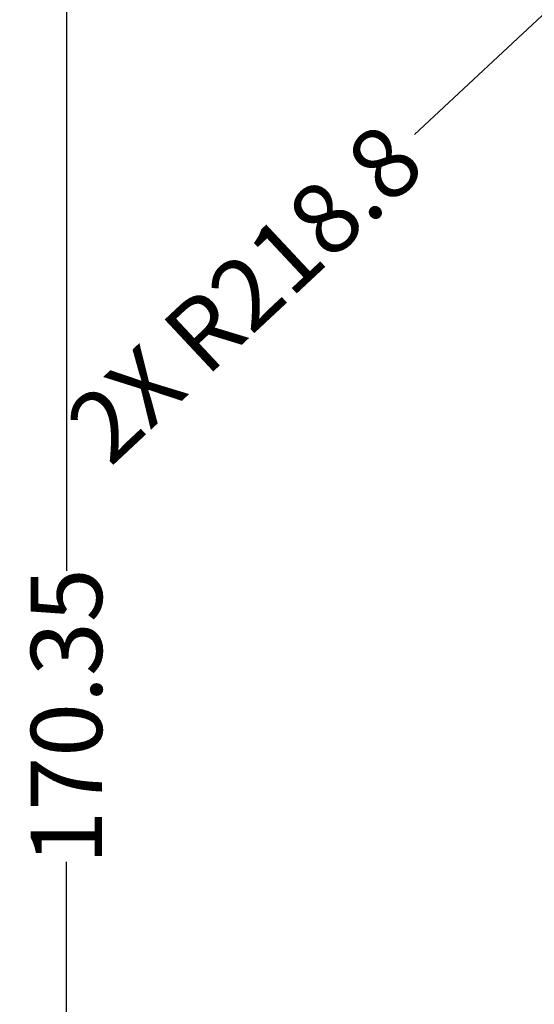
# Model space of a CAD drawing. Units: millimetres. Extents: x 0 to 2267, y 0 to 1823.
# Tile 4 of 256: x 1327 to 1378, y 1174 to 1271. Entities that reach past the tile are written whole.
import ezdxf

# ---------------------------------------------------------------- set-up
doc = ezdxf.new("R2010")
doc.units = ezdxf.units.MM
doc.header["$MEASUREMENT"] = 0
doc.layers.add('M-DIMS', color=2, linetype='Continuous', lineweight=25)
doc.styles.get("Standard").update_dxf_attribs({"font": 'arial.ttf'})
doc.dimstyles.get("Standard").update_dxf_attribs({"dimtxt": 7, "dimasz": 4, "dimexe": 0.18, "dimexo": 0.0625, "dimgap": 0.09, "dimtad": 0, "dimdec": 0, "dimzin": 0, "dimdsep": 46, "dimtxsty": 'Standard', "dimcen": 0.09, "dimadec": 0, "dimazin": 0, "dimtfac": 1, "dimtdec": 0, "dimtofl": 0, "dimtmove": 0, "dimatfit": 3, "dimfxl": 1, "dimtolj": 1, "dimtzin": 0, "dimarcsym": 0})

# ---------------------------------------------------------------- blocks, each defined once
blk = doc.blocks.new('*D10')
at = {"layer": 'Defpoints', "color": 0, "transparency": 16777216}
for p in [(1332.087, 1287.766), (1505.929, 1287.766), (1505.929, 1117.417)]:
    blk.add_point(p, dxfattribs=at)
at = {"layer": 'M-DIMS', "color": 0, "lineweight": -2, "transparency": 16777216}
for p, q in [((1505.866, 1287.766), (1331.907, 1287.766)), ((1332.087, 1283.766), (1332.087, 1216.908)), ((1332.087, 1121.417), (1332.087, 1188.275)), ((1505.866, 1117.417), (1331.907, 1117.417))]:
    blk.add_line(p, q, dxfattribs=at)
at = {"layer": 'M-DIMS', "color": 0, "transparency": 16777216}
for points in [[(1331.42, 1283.766), (1332.753, 1283.766), (1332.087, 1287.766)], [(1331.42, 1121.417), (1332.753, 1121.417), (1332.087, 1117.417)]]:
    blk.add_solid(points, dxfattribs=at)
at = {"layer": 'M-DIMS', "color": 0, "transparency": 16777216, "insert": (1332.087, 1202.591), "char_height": 7, "attachment_point": 5, "rotation": 90}
blk.add_mtext('\\A1;170.35', dxfattribs=at)
blk = doc.blocks.new('*D19')
at = {"layer": 'Defpoints', "color": 0, "transparency": 16777216}
for p in [(1605.34, 1483.304), (1445.529, 1333.885)]:
    blk.add_point(p, dxfattribs=at)
at = {"layer": 'M-DIMS', "color": 0, "lineweight": -2, "transparency": 16777216}
for p, q in [((1605.25, 1483.304), (1605.43, 1483.304)), ((1605.34, 1483.214), (1605.34, 1483.394)), ((1366.324, 1259.831), (1442.607, 1331.153))]:
    blk.add_line(p, q, dxfattribs=at)
at = {"layer": 'M-DIMS', "color": 0, "transparency": 16777216}
blk.add_solid([(1442.152, 1331.64), (1443.063, 1330.666), (1445.529, 1333.885)], dxfattribs=at)
at = {"layer": 'M-DIMS', "color": 0, "transparency": 16777216, "insert": (1349.643, 1244.233), "char_height": 7, "attachment_point": 5, "rotation": 43.07533}
blk.add_mtext('\\A1;2X R218.8', dxfattribs=at)

msp = doc.modelspace()

# ---------------------------------------------------------------- dimensions: what is measured, and where the dimension line sits
at = {"layer": 'M-DIMS'}
dim = msp.add_radius_dim(center=(1605.34, 1483.304), mpoint=(1445.529, 1333.885), text='2X <>', dimstyle='Standard', override={"dimdec": 1, "dimlfac": 1, "dimrnd": 0, "dimzin": 0, "dimdsep": 46, "dimlunit": 2}, dxfattribs=at)
dim.commit()
dim.dimension.update_dxf_attribs({"geometry": '*D19', "text_midpoint": (1349.643, 1244.233), "dimtype": 164})
dim = msp.add_linear_dim(base=(1332.087, 1287.766), p1=(1505.929, 1117.417), p2=(1505.929, 1287.766), angle=90, dimstyle='Standard', override={"dimdec": 2, "dimlfac": 1, "dimrnd": 0, "dimzin": 0, "dimdsep": 46, "dimlunit": 2}, dxfattribs=at)
dim.commit()
dim.dimension.update_dxf_attribs({"geometry": '*D10', "text_midpoint": (1332.087, 1202.591)})

doc.saveas('drawing.dxf')
